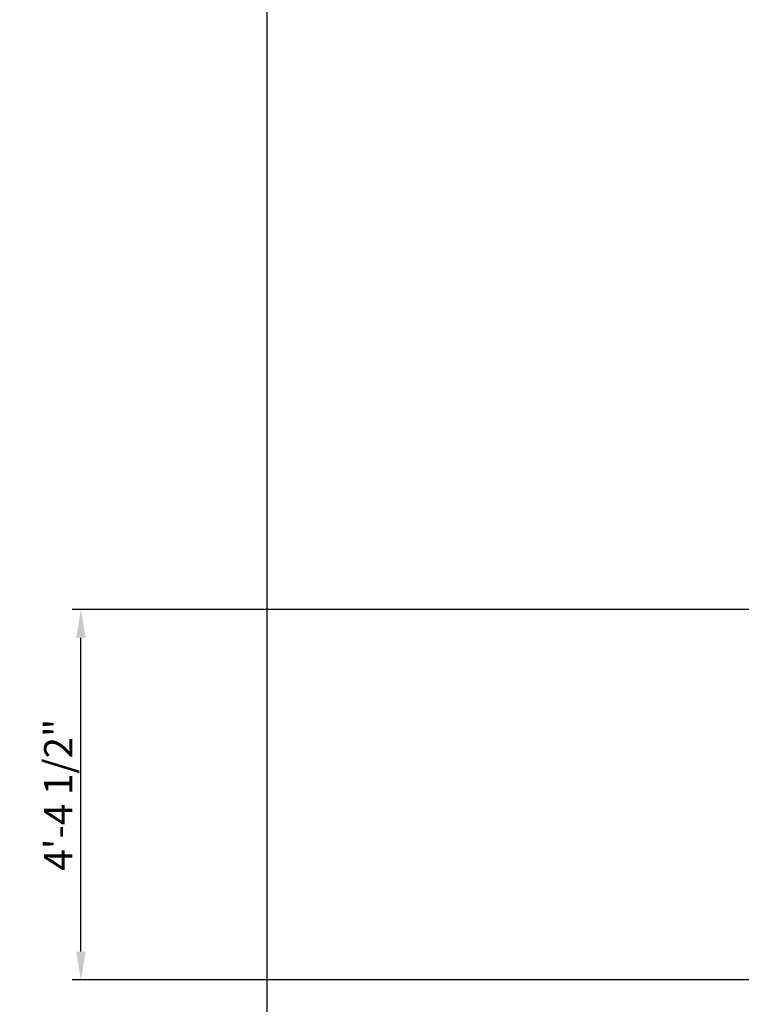
# Model space of a CAD drawing. Units: inches. Extents: x 2091 to 2899, y 967 to 2217.
# Tile 42 of 256: x 2091 to 2193, y 1096 to 1236. Entities that reach past the tile are written whole.
import ezdxf

# ---------------------------------------------------------------- set-up
doc = ezdxf.new("R2010")
doc.units = ezdxf.units.IN
doc.layers.add('A-ANNO-DIMS', color=2, linetype='Continuous', lineweight=18)
doc.styles.get("Standard").update_dxf_attribs({"font": 'arial.ttf'})
doc.dimstyles.new('ISO-25', dxfattribs={"dimtxt": 4, "dimasz": 4, "dimexe": 1.25, "dimexo": 0.625, "dimtad": 1, "dimdec": 0, "dimlunit": 3, "dimtxsty": 'Standard', "dimcen": 2.5, "dimadec": 0, "dimazin": 0, "dimtfac": 1, "dimtdec": 0, "dimtmove": 0, "dimatfit": 3, "dimfxl": 1, "dimarcsym": 0})

# ---------------------------------------------------------------- blocks, each defined once
blk = doc.blocks.new('*D32')
at = {"layer": 'A-ANNO-DIMS', "color": 0, "lineweight": -2, "transparency": 16777216}
for p, q in [((2178.68, 2050.68), (2124.59, 2050.68)), ((2125.84, 2046.68), (2125.84, 1094.68)), ((2178.68, 1090.68), (2124.59, 1090.68))]:
    blk.add_line(p, q, dxfattribs=at)
at = {"layer": 'A-ANNO-DIMS', "color": 0, "transparency": 16777216}
for points in [[(2125.18, 2046.68), (2126.51, 2046.68), (2125.84, 2050.68)], [(2125.18, 1094.68), (2126.51, 1094.68), (2125.84, 1090.68)]]:
    blk.add_solid(points, dxfattribs=at)
at = {"layer": 'Defpoints', "color": 0, "transparency": 16777216}
for p in [(2179.3, 2050.68), (2125.84, 1090.68), (2179.3, 1090.68)]:
    blk.add_point(p, dxfattribs=at)
at = {"layer": 'A-ANNO-DIMS', "color": 0, "transparency": 16777216, "insert": (2123.18, 1570.68), "char_height": 4, "attachment_point": 5, "rotation": 90}
blk.add_mtext("80'", dxfattribs=at)
blk = doc.blocks.new('*D91')
at = {"layer": 'A-ANNO-DIMS', "color": 0, "lineweight": -2, "transparency": 16777216}
for p, q in [((2211.65, 1152.25), (2098.31, 1152.25)), ((2099.56, 1103.92), (2099.56, 1148.25)), ((2211.52, 1099.92), (2098.31, 1099.92))]:
    blk.add_line(p, q, dxfattribs=at)
at = {"layer": 'A-ANNO-DIMS', "color": 0, "transparency": 16777216}
for points in [[(2098.89, 1148.25), (2100.23, 1148.25), (2099.56, 1152.25)], [(2098.89, 1103.92), (2100.23, 1103.92), (2099.56, 1099.92)]]:
    blk.add_solid(points, dxfattribs=at)
at = {"layer": 'Defpoints', "color": 0, "transparency": 16777216}
for p in [(2099.56, 1152.25), (2212.28, 1152.25), (2212.14, 1099.92)]:
    blk.add_point(p, dxfattribs=at)
at = {"layer": 'A-ANNO-DIMS', "color": 0, "transparency": 16777216, "insert": (2096.87, 1126.08), "char_height": 4, "attachment_point": 5, "rotation": 90}
blk.add_mtext('4\'-4 1/2"', dxfattribs=at)

msp = doc.modelspace()

# ---------------------------------------------------------------- dimensions: what is measured, and where the dimension line sits
at = {"layer": 'A-ANNO-DIMS'}
for base, p1, p2, override, picture, middle in [((2125.84, 1090.68), (2179.3, 2050.68), (2179.3, 1090.68), {"dimclrd": 0, "dimclre": 0, "dimclrt": 0}, '*D32', (2123.18, 1570.68)), ((2099.56, 1152.25), (2212.14, 1099.92), (2212.28, 1152.25), {"dimdec": 1, "dimlfac": 1, "dimrnd": 0, "dimzin": 1, "dimdsep": 46, "dimlunit": 4, "dimfrac": 2}, '*D91', (2096.87, 1126.08))]:
    dim = msp.add_linear_dim(base=base, p1=p1, p2=p2, angle=90, dimstyle='ISO-25', override=override, dxfattribs=at)
    dim.commit()
    dim.dimension.update_dxf_attribs({"geometry": picture, "text_midpoint": middle})

doc.saveas('drawing.dxf')
